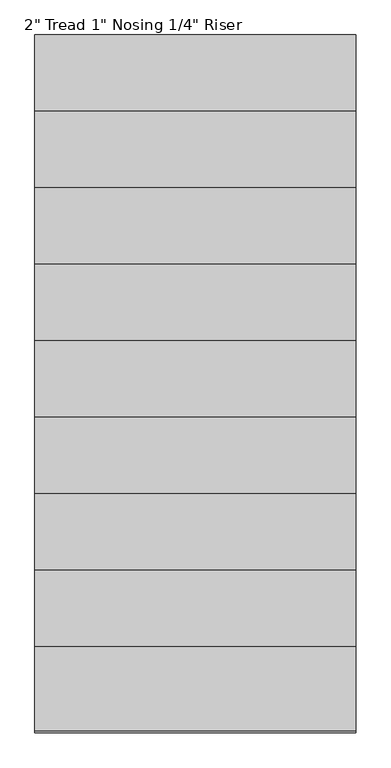
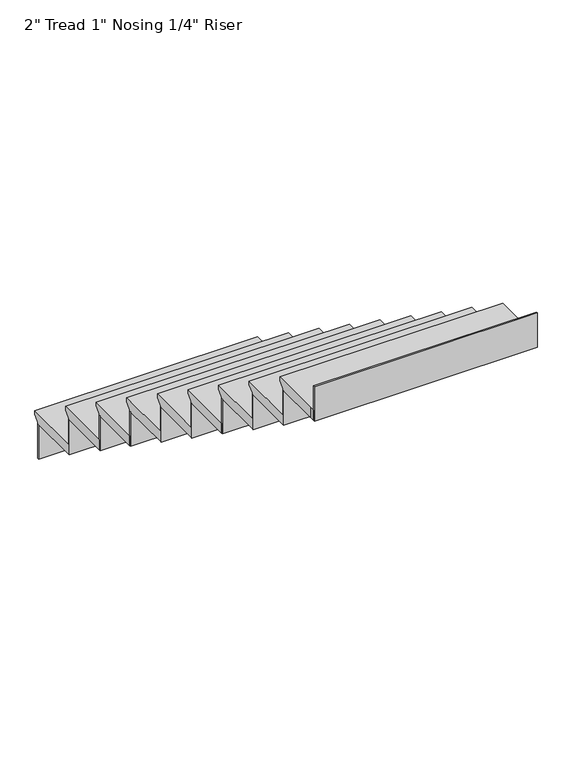
"""IFC4 building model written with IfcOpenShell, lengths in millimetres: stair flight geometry."""

from ifc_helpers import new_model, si_unit, origin, place, context, project, spatial, faceted_brep, source, transform, mapped, element, save


def stair_flight_6a237a90(model_context):
    return source(origin(), model_context, "Body", "Brep", [
        faceted_brep([(17678.7916032, 5155.1241878, 1032.51), (17678.7916032, 5155.1241878, 1051.56), (18745.5916032, 5155.1241878, 1051.56), (18745.5916032, 5155.1241878, 1032.51), (17678.7916032, 5129.7241878, 1007.11), (18745.5916032, 5129.7241878, 1007.11), (17678.7916032, 4875.7241878, 1051.56), (18745.5916032, 4875.7241878, 1051.56), (18745.5916032, 5129.7241878, 1000.76), (18745.5916032, 4875.7241878, 1000.76), (17678.7916032, 4875.7241878, 1000.76), (17678.7916032, 5129.7241878, 1000.76)], [[[0, 1, 2, 3]], [[4, 0, 3, 5]], [[2, 1, 6, 7]], [[8, 9, 10, 11]], [[2, 7, 9, 8, 5, 3]], [[8, 11, 4, 5]], [[6, 1, 0, 4, 11, 10]], [[7, 6, 10, 9]]]),
        faceted_brep([(17678.7916032, 5129.7241878, 1000.76), (17678.7916032, 5129.7241878, 825.5), (17678.7916032, 5123.3741878, 825.5), (17678.7916032, 5123.3741878, 1000.76), (18745.5916032, 5129.7241878, 1000.76), (18745.5916032, 5123.3741878, 1000.76), (18745.5916032, 5123.3741878, 825.5), (18745.5916032, 5129.7241878, 825.5)], [[[0, 1, 2, 3]], [[4, 5, 6, 7]], [[1, 0, 4, 7]], [[2, 1, 7, 6]], [[3, 2, 6, 5]], [[0, 3, 5, 4]]]),
        faceted_brep([(17678.7916032, 4875.7241878, 1176.02), (17678.7916032, 4875.7241878, 1000.76), (17678.7916032, 4869.3741878, 1000.76), (17678.7916032, 4869.3741878, 1176.02), (18745.5916032, 4875.7241878, 1176.02), (18745.5916032, 4869.3741878, 1176.02), (18745.5916032, 4869.3741878, 1000.76), (18745.5916032, 4875.7241878, 1000.76)], [[[0, 1, 2, 3]], [[4, 5, 6, 7]], [[1, 0, 4, 7]], [[2, 1, 7, 6]], [[3, 2, 6, 5]], [[0, 3, 5, 4]]]),
        faceted_brep([(18745.5916032, 4901.1241878, 1226.82), (17678.7916032, 4901.1241878, 1226.82), (17678.7916032, 4621.7241878, 1226.82), (18745.5916032, 4621.7241878, 1226.82), (18745.5916032, 4875.7241878, 1176.02), (18745.5916032, 4621.7241878, 1176.02), (17678.7916032, 4621.7241878, 1176.02), (17678.7916032, 4875.7241878, 1176.02), (18745.5916032, 4875.7241878, 1182.37), (18745.5916032, 4901.1241878, 1207.77), (17678.7916032, 4875.7241878, 1182.37), (17678.7916032, 4901.1241878, 1207.77)], [[[0, 1, 2, 3]], [[4, 5, 6, 7]], [[0, 3, 5, 4, 8, 9]], [[4, 7, 10, 8]], [[2, 1, 11, 10, 7, 6]], [[3, 2, 6, 5]], [[11, 1, 0, 9]], [[10, 11, 9, 8]]]),
        faceted_brep([(17678.7916032, 4621.7241878, 1351.28), (17678.7916032, 4621.7241878, 1176.02), (17678.7916032, 4615.3741878, 1176.02), (17678.7916032, 4615.3741878, 1351.28), (18745.5916032, 4621.7241878, 1351.28), (18745.5916032, 4615.3741878, 1351.28), (18745.5916032, 4615.3741878, 1176.02), (18745.5916032, 4621.7241878, 1176.02)], [[[0, 1, 2, 3]], [[4, 5, 6, 7]], [[1, 0, 4, 7]], [[2, 1, 7, 6]], [[3, 2, 6, 5]], [[0, 3, 5, 4]]]),
        faceted_brep([(18745.5916032, 4647.1241878, 1402.08), (17678.7916032, 4647.1241878, 1402.08), (17678.7916032, 4367.7241878, 1402.08), (18745.5916032, 4367.7241878, 1402.08), (18745.5916032, 4621.7241878, 1351.28), (18745.5916032, 4367.7241878, 1351.28), (17678.7916032, 4367.7241878, 1351.28), (17678.7916032, 4621.7241878, 1351.28), (18745.5916032, 4621.7241878, 1357.63), (18745.5916032, 4647.1241878, 1383.03), (17678.7916032, 4621.7241878, 1357.63), (17678.7916032, 4647.1241878, 1383.03)], [[[0, 1, 2, 3]], [[4, 5, 6, 7]], [[0, 3, 5, 4, 8, 9]], [[4, 7, 10, 8]], [[2, 1, 11, 10, 7, 6]], [[3, 2, 6, 5]], [[11, 1, 0, 9]], [[10, 11, 9, 8]]]),
        faceted_brep([(17678.7916032, 4367.7241878, 1526.54), (17678.7916032, 4367.7241878, 1351.28), (17678.7916032, 4361.3741878, 1351.28), (17678.7916032, 4361.3741878, 1526.54), (18745.5916032, 4367.7241878, 1526.54), (18745.5916032, 4361.3741878, 1526.54), (18745.5916032, 4361.3741878, 1351.28), (18745.5916032, 4367.7241878, 1351.28)], [[[0, 1, 2, 3]], [[4, 5, 6, 7]], [[1, 0, 4, 7]], [[2, 1, 7, 6]], [[3, 2, 6, 5]], [[0, 3, 5, 4]]]),
        faceted_brep([(18745.5916032, 4393.1241878, 1577.34), (17678.7916032, 4393.1241878, 1577.34), (17678.7916032, 4113.7241878, 1577.34), (18745.5916032, 4113.7241878, 1577.34), (18745.5916032, 4367.7241878, 1526.54), (18745.5916032, 4113.7241878, 1526.54), (17678.7916032, 4113.7241878, 1526.54), (17678.7916032, 4367.7241878, 1526.54), (18745.5916032, 4367.7241878, 1532.89), (18745.5916032, 4393.1241878, 1558.29), (17678.7916032, 4367.7241878, 1532.89), (17678.7916032, 4393.1241878, 1558.29)], [[[0, 1, 2, 3]], [[4, 5, 6, 7]], [[0, 3, 5, 4, 8, 9]], [[4, 7, 10, 8]], [[2, 1, 11, 10, 7, 6]], [[3, 2, 6, 5]], [[11, 1, 0, 9]], [[10, 11, 9, 8]]]),
        faceted_brep([(17678.7916032, 4113.7241878, 1701.8), (17678.7916032, 4113.7241878, 1526.54), (17678.7916032, 4107.3741878, 1526.54), (17678.7916032, 4107.3741878, 1701.8), (18745.5916032, 4113.7241878, 1701.8), (18745.5916032, 4107.3741878, 1701.8), (18745.5916032, 4107.3741878, 1526.54), (18745.5916032, 4113.7241878, 1526.54)], [[[0, 1, 2, 3]], [[4, 5, 6, 7]], [[1, 0, 4, 7]], [[2, 1, 7, 6]], [[3, 2, 6, 5]], [[0, 3, 5, 4]]]),
        faceted_brep([(18745.5916032, 4139.1241878, 1752.6), (17678.7916032, 4139.1241878, 1752.6), (17678.7916032, 3859.7241878, 1752.6), (18745.5916032, 3859.7241878, 1752.6), (18745.5916032, 4113.7241878, 1701.8), (18745.5916032, 3859.7241878, 1701.8), (17678.7916032, 3859.7241878, 1701.8), (17678.7916032, 4113.7241878, 1701.8), (18745.5916032, 4113.7241878, 1708.15), (18745.5916032, 4139.1241878, 1733.55), (17678.7916032, 4113.7241878, 1708.15), (17678.7916032, 4139.1241878, 1733.55)], [[[0, 1, 2, 3]], [[4, 5, 6, 7]], [[0, 3, 5, 4, 8, 9]], [[4, 7, 10, 8]], [[2, 1, 11, 10, 7, 6]], [[3, 2, 6, 5]], [[11, 1, 0, 9]], [[10, 11, 9, 8]]]),
        faceted_brep([(17678.7916032, 3859.7241878, 1877.06), (17678.7916032, 3859.7241878, 1701.8), (17678.7916032, 3853.3741878, 1701.8), (17678.7916032, 3853.3741878, 1877.06), (18745.5916032, 3859.7241878, 1877.06), (18745.5916032, 3853.3741878, 1877.06), (18745.5916032, 3853.3741878, 1701.8), (18745.5916032, 3859.7241878, 1701.8)], [[[0, 1, 2, 3]], [[4, 5, 6, 7]], [[1, 0, 4, 7]], [[2, 1, 7, 6]], [[3, 2, 6, 5]], [[0, 3, 5, 4]]]),
        faceted_brep([(18745.5916032, 3885.1241878, 1927.86), (17678.7916032, 3885.1241878, 1927.86), (17678.7916032, 3605.7241878, 1927.86), (18745.5916032, 3605.7241878, 1927.86), (18745.5916032, 3859.7241878, 1877.06), (18745.5916032, 3605.7241878, 1877.06), (17678.7916032, 3605.7241878, 1877.06), (17678.7916032, 3859.7241878, 1877.06), (18745.5916032, 3859.7241878, 1883.41), (18745.5916032, 3885.1241878, 1908.81), (17678.7916032, 3859.7241878, 1883.41), (17678.7916032, 3885.1241878, 1908.81)], [[[0, 1, 2, 3]], [[4, 5, 6, 7]], [[0, 3, 5, 4, 8, 9]], [[4, 7, 10, 8]], [[2, 1, 11, 10, 7, 6]], [[3, 2, 6, 5]], [[11, 1, 0, 9]], [[10, 11, 9, 8]]]),
        faceted_brep([(17678.7916032, 3605.7241878, 2052.32), (17678.7916032, 3605.7241878, 1877.06), (17678.7916032, 3599.3741878, 1877.06), (17678.7916032, 3599.3741878, 2052.32), (18745.5916032, 3605.7241878, 2052.32), (18745.5916032, 3599.3741878, 2052.32), (18745.5916032, 3599.3741878, 1877.06), (18745.5916032, 3605.7241878, 1877.06)], [[[0, 1, 2, 3]], [[4, 5, 6, 7]], [[1, 0, 4, 7]], [[2, 1, 7, 6]], [[3, 2, 6, 5]], [[0, 3, 5, 4]]]),
        faceted_brep([(18745.5916032, 3631.1241878, 2103.12), (17678.7916032, 3631.1241878, 2103.12), (17678.7916032, 3351.7241878, 2103.12), (18745.5916032, 3351.7241878, 2103.12), (18745.5916032, 3605.7241878, 2052.32), (18745.5916032, 3351.7241878, 2052.32), (17678.7916032, 3351.7241878, 2052.32), (17678.7916032, 3605.7241878, 2052.32), (18745.5916032, 3605.7241878, 2058.67), (18745.5916032, 3631.1241878, 2084.07), (17678.7916032, 3605.7241878, 2058.67), (17678.7916032, 3631.1241878, 2084.07)], [[[0, 1, 2, 3]], [[4, 5, 6, 7]], [[0, 3, 5, 4, 8, 9]], [[4, 7, 10, 8]], [[2, 1, 11, 10, 7, 6]], [[3, 2, 6, 5]], [[11, 1, 0, 9]], [[10, 11, 9, 8]]]),
        faceted_brep([(17678.7916032, 3351.7241878, 2227.58), (17678.7916032, 3351.7241878, 2052.32), (17678.7916032, 3345.3741878, 2052.32), (17678.7916032, 3345.3741878, 2227.58), (18745.5916032, 3351.7241878, 2227.58), (18745.5916032, 3345.3741878, 2227.58), (18745.5916032, 3345.3741878, 2052.32), (18745.5916032, 3351.7241878, 2052.32)], [[[0, 1, 2, 3]], [[4, 5, 6, 7]], [[1, 0, 4, 7]], [[2, 1, 7, 6]], [[3, 2, 6, 5]], [[0, 3, 5, 4]]]),
        faceted_brep([(18745.5916032, 3377.1241878, 2278.38), (17678.7916032, 3377.1241878, 2278.38), (17678.7916032, 3097.7241878, 2278.38), (18745.5916032, 3097.7241878, 2278.38), (18745.5916032, 3351.7241878, 2227.58), (18745.5916032, 3097.7241878, 2227.58), (17678.7916032, 3097.7241878, 2227.58), (17678.7916032, 3351.7241878, 2227.58), (18745.5916032, 3351.7241878, 2233.93), (18745.5916032, 3377.1241878, 2259.33), (17678.7916032, 3351.7241878, 2233.93), (17678.7916032, 3377.1241878, 2259.33)], [[[0, 1, 2, 3]], [[4, 5, 6, 7]], [[0, 3, 5, 4, 8, 9]], [[4, 7, 10, 8]], [[2, 1, 11, 10, 7, 6]], [[3, 2, 6, 5]], [[11, 1, 0, 9]], [[10, 11, 9, 8]]]),
        faceted_brep([(17678.7916032, 2843.7241878, 2578.1), (17678.7916032, 2843.7241878, 2402.84), (17678.7916032, 2837.3741878, 2402.84), (17678.7916032, 2837.3741878, 2578.1), (18745.5916032, 2843.7241878, 2578.1), (18745.5916032, 2837.3741878, 2578.1), (18745.5916032, 2837.3741878, 2402.84), (18745.5916032, 2843.7241878, 2402.84)], [[[0, 1, 2, 3]], [[4, 5, 6, 7]], [[1, 0, 4, 7]], [[2, 1, 7, 6]], [[3, 2, 6, 5]], [[0, 3, 5, 4]]]),
        faceted_brep([(17678.7916032, 3097.7241878, 2402.84), (17678.7916032, 3097.7241878, 2227.58), (17678.7916032, 3091.3741878, 2227.58), (17678.7916032, 3091.3741878, 2402.84), (18745.5916032, 3097.7241878, 2402.84), (18745.5916032, 3091.3741878, 2402.84), (18745.5916032, 3091.3741878, 2227.58), (18745.5916032, 3097.7241878, 2227.58)], [[[0, 1, 2, 3]], [[4, 5, 6, 7]], [[1, 0, 4, 7]], [[2, 1, 7, 6]], [[3, 2, 6, 5]], [[0, 3, 5, 4]]]),
        faceted_brep([(18745.5916032, 2843.7241878, 2453.64), (18745.5916032, 2869.1241878, 2453.64), (18745.5916032, 3123.1241878, 2453.64), (17678.7916032, 3123.1241878, 2453.64), (17678.7916032, 2869.1241878, 2453.64), (17678.7916032, 2843.7241878, 2453.64), (18745.5916032, 2869.1241878, 2402.84), (18745.5916032, 2843.7241878, 2402.84), (17678.7916032, 2843.7241878, 2402.84), (17678.7916032, 2869.1241878, 2402.84), (17678.7916032, 3097.7241878, 2402.84), (18745.5916032, 3097.7241878, 2402.84), (18745.5916032, 3097.7241878, 2409.19), (18745.5916032, 3123.1241878, 2434.59), (17678.7916032, 3097.7241878, 2409.19), (17678.7916032, 3123.1241878, 2434.59)], [[[0, 1, 2, 3, 4, 5]], [[6, 7, 8, 9, 10, 11]], [[1, 0, 7, 6]], [[2, 1, 6, 11, 12, 13]], [[11, 10, 14, 12]], [[4, 3, 15, 14, 10, 9]], [[5, 4, 9, 8]], [[0, 5, 8, 7]], [[15, 3, 2, 13]], [[14, 15, 13, 12]]]),
    ])


if __name__ == "__main__":
    model = new_model("IFC4")
    model_context = context("Model", 3, world=origin())
    ifc_project = project(units=[si_unit("LENGTHUNIT", "METRE", prefix="MILLI")], contexts=[model_context])
    site = spatial("IfcSite", under=ifc_project)
    building = spatial("IfcBuilding", under=site)
    placement = place(None, origin())
    stair_flight_shape = stair_flight_6a237a90(model_context)
    element("IfcStairFlight", 1, ObjectType="2\" Tread 1\" Nosing 1/4\" Riser", at=placement, inside=building, context=model_context, shape_type="MappedRepresentation", body=[
        mapped(stair_flight_shape, transform((0.0, 0.0, 0.0), x_axis=(1.0, 0.0, 0.0), y_axis=(0.0, 1.0, 0.0), z_axis=(0.0, 0.0, 1.0))),
    ])
    save(model, "model.ifc")
